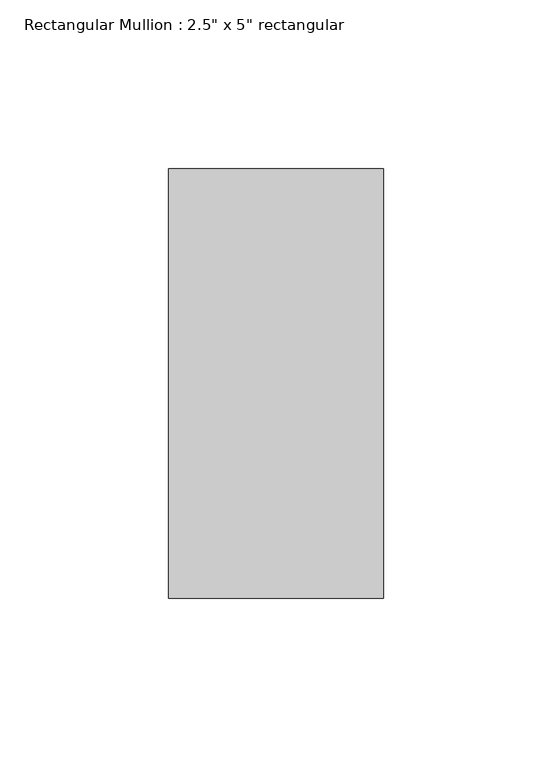
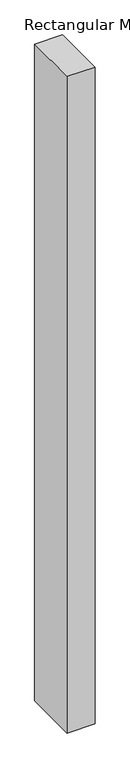
"""IFC4 building model written with IfcOpenShell, lengths in millimetres: member geometry."""

from ifc_helpers import new_model, si_unit, frame, origin, place, context, project, spatial, polyline, outline, extrude, source, transform, mapped, element, save


def member_9efbbc5c(model_context):
    return source(origin(), model_context, "Body", "SweptSolid", [
        extrude(outline(polyline([(0.0, 63.5), (0.0, -63.5), (-63.5, -63.5), (-63.5, 63.5), (0.0, 63.5)])), frame((0.0, 0.0, -1573.6725209), z_axis=(0.0, 0.0, 1.0), x_axis=(1.0, 0.0, 0.0)), (0.0, 0.0, 1.0), 1573.6725209),
    ])


if __name__ == "__main__":
    model = new_model("IFC4")
    model_context = context("Model", 3, world=origin())
    ifc_project = project(units=[si_unit("LENGTHUNIT", "METRE", prefix="MILLI")], contexts=[model_context])
    site = spatial("IfcSite", under=ifc_project)
    building = spatial("IfcBuilding", under=site)
    placement = place(None, origin())
    member_shape = member_9efbbc5c(model_context)
    element("IfcMember", 1, ObjectType="Rectangular Mullion : 2.5\" x 5\" rectangular", at=placement, inside=building, context=model_context, shape_type="MappedRepresentation", body=[
        mapped(member_shape, transform((0.0, 0.0, 0.0), x_axis=(1.0, 0.0, 0.0), y_axis=(0.0, 1.0, 0.0), z_axis=(0.0, 0.0, 1.0))),
    ])
    save(model, "model.ifc")

# Revit data of these elements
# Type "Rectangular Mullion : 2.5\" x 5\" rectangular"
#   built-in parameter 1007304 = 0.416667 (stored number, unit not read)
#   built-in parameter 1007301 = 0.104167 (stored number, unit not read)
#   built-in parameter 1007300 = 0.104167 (stored number, unit not read)
# Element 1 (IfcMember, "Rectangular Mullion : 2.5\" x 5\" rectangular")
#   Materials on its faces: "Aluminum"
# Materials
#   "Aluminum": class "Metal", colour RGB 247 247 247, transparency 0, Description = "Aluminum 6061", Cost = 0
